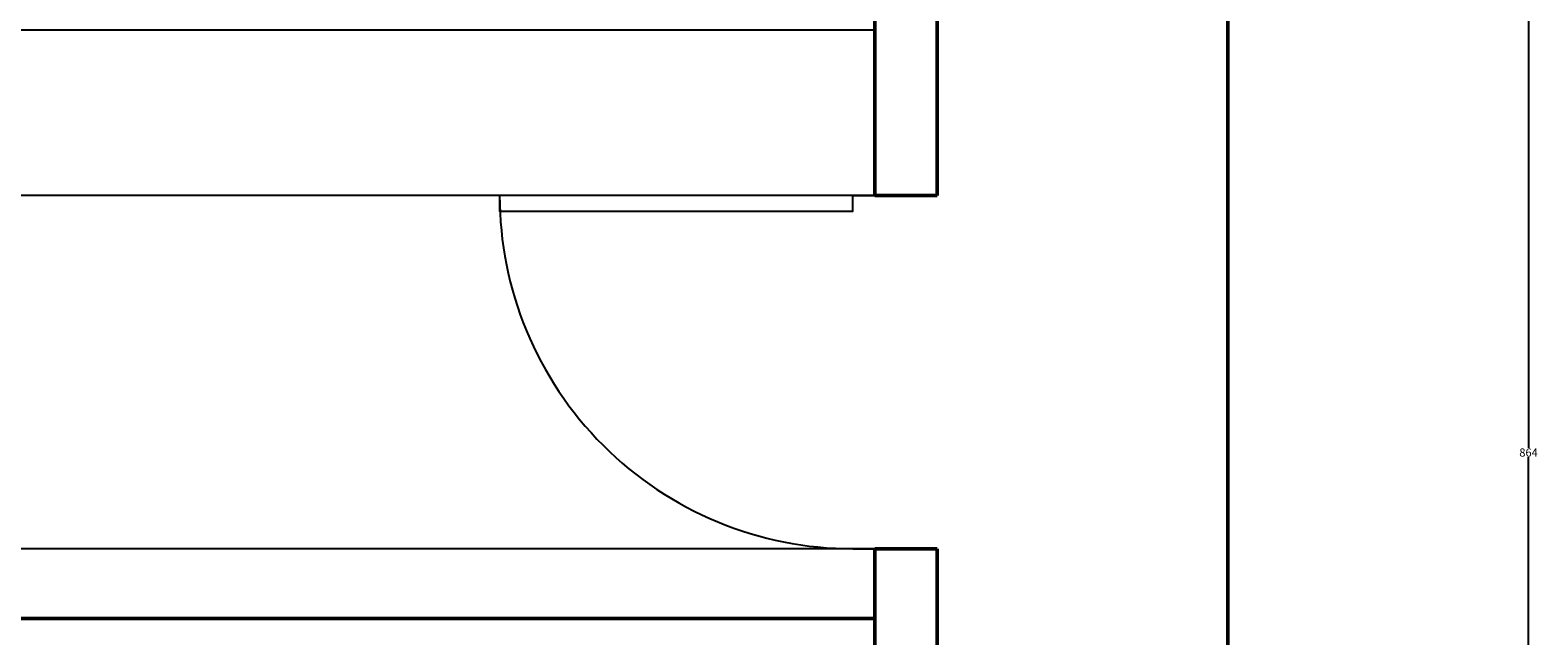
# Model space of a CAD drawing. Units: inches. Extents: x 3506 to 3958, y 1553 to 2506.
# Tile 11 of 16: x 3739 to 3957, y 2003 to 2090. Entities that reach past the tile are written whole.
import ezdxf

# ---------------------------------------------------------------- set-up
doc = ezdxf.new("R2010")
doc.units = ezdxf.units.IN
doc.header["$MEASUREMENT"] = 0
for name, color, linetype, lineweight in [('A-ANNO-DIMS', 2, 'Continuous', 18), ('A-WALL', 7, 'Continuous', 50), ('doors', 40, 'Continuous', 25)]:
    doc.layers.add(name, color=color, linetype=linetype, lineweight=lineweight)
doc.layers.add('A-WALL-PATT', color=251, linetype='Continuous', lineweight=13, true_color=0x636466)
doc.styles.get("Standard").update_dxf_attribs({"font": 'arial.ttf'})
doc.dimstyles.get("Standard").update_dxf_attribs({"dimtxt": 1.18, "dimasz": 0.68, "dimexe": 0.18, "dimexo": 0.0625, "dimgap": 0.09, "dimtad": 0, "dimtih": 1, "dimtoh": 1, "dimdec": 1, "dimzin": 0, "dimdsep": 46, "dimlunit": 3, "dimtxsty": 'Standard', "dimcen": 0.09, "dimadec": 0, "dimazin": 0, "dimtfac": 1, "dimtdec": 1, "dimtofl": 0, "dimtmove": 0, "dimatfit": 3, "dimfxl": 1, "dimtolj": 1, "dimtzin": 0, "dimarcsym": 0})

# ---------------------------------------------------------------- blocks, each defined once
blk = doc.blocks.new('*U12')
for p, q in [((0, 0), (0, 6)), ((40, 0), (40, 6))]:
    blk.add_line(p, q)
blk.add_lwpolyline([(0, 0), (0, -40), (1.75, -40), (1.75, 0)], close=True)
blk.add_arc((0, 0), 40, 270, 0)
blk = doc.blocks.new('*D39')
at = {"layer": 'A-ANNO-DIMS', "color": 0, "lineweight": -2, "transparency": 16777216}
for p, q in [((3911.79, 2461.39), (3955.36, 2461.39)), ((3955.18, 2460.71), (3955.18, 2030.09)), ((3955.18, 1598.07), (3955.18, 2028.7)), ((3911.79, 1597.39), (3955.36, 1597.39))]:
    blk.add_line(p, q, dxfattribs=at)
at = {"layer": 'A-ANNO-DIMS', "color": 0, "transparency": 16777216}
for points in [[(3955.07, 2460.71), (3955.29, 2460.71), (3955.18, 2461.39)], [(3955.07, 1598.07), (3955.29, 1598.07), (3955.18, 1597.39)]]:
    blk.add_solid(points, dxfattribs=at)
at = {"layer": 'Defpoints', "color": 0, "transparency": 16777216}
for p in [(3911.73, 2461.39), (3955.18, 2461.39), (3911.73, 1597.39)]:
    blk.add_point(p, dxfattribs=at)
at = {"layer": 'A-ANNO-DIMS', "color": 0, "transparency": 16777216, "insert": (3955.18, 2029.39), "char_height": 1.18, "attachment_point": 5}
blk.add_mtext('\\A1;864', dxfattribs=at)
blk = doc.blocks.new('*D60')
at = {"layer": 'A-ANNO-DIMS', "color": 0, "lineweight": -2, "transparency": 16777216}
for p, q in [((3860.67, 2066.52), (3508.1, 2066.52)), ((3508.28, 2065.84), (3508.28, 2041.7)), ((3508.28, 2016.17), (3508.28, 2040.31)), ((3860.67, 2015.49), (3508.1, 2015.49))]:
    blk.add_line(p, q, dxfattribs=at)
at = {"layer": 'A-ANNO-DIMS', "color": 0, "transparency": 16777216}
for points in [[(3508.17, 2065.84), (3508.39, 2065.84), (3508.28, 2066.52)], [(3508.17, 2016.17), (3508.39, 2016.17), (3508.28, 2015.49)]]:
    blk.add_solid(points, dxfattribs=at)
at = {"layer": 'Defpoints', "color": 0, "transparency": 16777216}
for p in [(3860.73, 2066.52), (3508.28, 2015.49), (3860.73, 2015.49)]:
    blk.add_point(p, dxfattribs=at)
at = {"layer": 'A-ANNO-DIMS', "color": 0, "transparency": 16777216, "insert": (3508.28, 2041), "char_height": 1.18, "attachment_point": 5}
blk.add_mtext('\\A1;51.03', dxfattribs=at)
blk = doc.blocks.new('*D61')
at = {"layer": 'A-ANNO-DIMS', "color": 0, "lineweight": -2, "transparency": 16777216}
for p, q in [((3860.67, 2090.43), (3508.1, 2090.43)), ((3508.28, 2089.75), (3508.28, 2079.17)), ((3508.28, 2067.2), (3508.28, 2077.78)), ((3860.67, 2066.52), (3508.1, 2066.52))]:
    blk.add_line(p, q, dxfattribs=at)
at = {"layer": 'A-ANNO-DIMS', "color": 0, "transparency": 16777216}
for points in [[(3508.17, 2089.75), (3508.39, 2089.75), (3508.28, 2090.43)], [(3508.17, 2067.2), (3508.39, 2067.2), (3508.28, 2066.52)]]:
    blk.add_solid(points, dxfattribs=at)
at = {"layer": 'Defpoints', "color": 0, "transparency": 16777216}
for p in [(3860.73, 2090.43), (3508.28, 2066.52), (3860.73, 2066.52)]:
    blk.add_point(p, dxfattribs=at)
at = {"layer": 'A-ANNO-DIMS', "color": 0, "transparency": 16777216, "insert": (3508.28, 2078.48), "char_height": 1.18, "attachment_point": 5}
blk.add_mtext('\\A1;23.92', dxfattribs=at)

msp = doc.modelspace()

# ---------------------------------------------------------------- hatches: boundary and pattern name
at = {"layer": 'A-WALL-PATT'}
h = msp.add_hatch(dxfattribs=at)
h.set_pattern_fill('ANSI31', color=256)
h.paths.add_polyline_path([(3911.7302, 2461.3942), (3551.7302, 2461.3942), (3551.7302, 2152.516), (3560.7302, 2152.516), (3560.7302, 2116.516), (3551.7302, 2116.516), (3551.7302, 1920.5711), (3556.2302, 1920.5711), (3560.7302, 1920.5711), (3560.7302, 2000.3942), (3692.7302, 2000.3942), (3692.7302, 1997.3942), (3697.7302, 1997.3942), (3697.7302, 2000.3942), (3771.7302, 2000.3942), (3771.7302, 1997.3942), (3776.7302, 1997.3942), (3776.7302, 1997.7206), (3778.5802, 1997.7206), (3807.5802, 1997.7206), (3807.5802, 1996.4519), (3778.5802, 1996.4519), (3778.5802, 1997.7206), (3776.7302, 1997.7206), (3776.7302, 1997.3942), (3771.7302, 1997.3942), (3771.7302, 2000.3942), (3697.7302, 2000.3942), (3697.7302, 1997.3942), (3692.7302, 1997.3942), (3689.8302, 1997.3942), (3689.8302, 1995.8192), (3653.8302, 1995.8192), (3653.8302, 1997.3942), (3689.8302, 1997.3942), (3692.7302, 1997.3942), (3692.7302, 2000.3942), (3560.7302, 2000.3942), (3560.7302, 1920.5711), (3551.7302, 1920.5711), (3551.7302, 1884.5711), (3551.7302, 1597.3942), (3911.7302, 1597.3942)], flags=17)
h.paths.add_polyline_path([(3596.7302, 2005.3942), (3596.7302, 2057.3035, -0.38730371), (3569.1778, 2085), (3569.15, 2085), (3569.15, 2086.2688), (3598.15, 2086.2688), (3598.15, 2085), (3569.1778, 2085, 0.38730371), (3596.7302, 2057.3035), (3596.7302, 2057.3942), (3601.7302, 2057.3942), (3601.7302, 2055.3942), (3630.7302, 2055.3942), (3630.7302, 2034.3942), (3694.7302, 2034.3942), (3694.7302, 2053.3942), (3699.7302, 2053.3942), (3699.7302, 2005.3942), (3860.7302, 2005.3942), (3860.7302, 2173.3942), (3771.7302, 2173.3942), (3771.7302, 2194.3942), (3776.7302, 2194.3942), (3776.7302, 2178.3942), (3860.7302, 2178.3942), (3860.7302, 2231.3942), (3601.7302, 2231.3942), (3601.7302, 2241.426), (3596.7302, 2241.426), (3596.7302, 2231.3942), (3560.7302, 2231.3942), (3560.7302, 2315.3942), (3596.7302, 2315.3942), (3596.7302, 2312.3942), (3601.7302, 2312.3942), (3601.7302, 2315.3942), (3697.7302, 2315.3942), (3697.7302, 2413.3942), (3692.7302, 2413.3942), (3692.7302, 2320.3942), (3560.7302, 2320.3942), (3560.7302, 2452.3942), (3692.7302, 2452.3942), (3692.7302, 2449.3942), (3697.7302, 2449.3942), (3697.7302, 2452.3942), (3771.7302, 2452.3942), (3771.7302, 2449.3942), (3776.7302, 2449.3942), (3776.7302, 2452.3942), (3860.7302, 2452.3942), (3860.7302, 2437.2075), (3865.2302, 2437.2075), (3865.2302, 2413.2075), (3860.7302, 2413.2075), (3860.7302, 2367.6976), (3865.2302, 2367.6976), (3869.7302, 2367.6976), (3869.7302, 2319.6976), (3860.7302, 2319.6976), (3860.7302, 2211.6248), (3869.7302, 2211.6248), (3869.7302, 2187.6248), (3860.7302, 2187.6248), (3860.7302, 2138.4346), (3865.2302, 2138.4346), (3869.7302, 2138.4346), (3869.7302, 2090.4346), (3860.7302, 2090.4346), (3860.7302, 1985.8449), (3869.7302, 1985.8449), (3869.7302, 1961.8449), (3860.7302, 1961.8449), (3860.7302, 1897.0756), (3865.2302, 1897.0756), (3869.7302, 1897.0756), (3869.7302, 1849.0756), (3860.7302, 1849.0756), (3860.7302, 1847.8112), (3860.7302, 1779.3942), (3596.7302, 1779.3942), (3596.7302, 1831.3942), (3601.7302, 1831.3942), (3601.7302, 1828.3942), (3630.7302, 1828.3942), (3630.7302, 1808.3942), (3691.7302, 1808.3942), (3691.7302, 1815.3942), (3696.7302, 1815.3942), (3696.7302, 1779.3942), (3860.7302, 1779.3942), (3860.7302, 1947.3942), (3771.7302, 1947.3942), (3771.7302, 1968.3942), (3776.7302, 1968.3942), (3776.7302, 1952.3942), (3860.7302, 1952.3942), (3860.7302, 2005.3942)], flags=0)
h.paths.add_polyline_path([(3596.7302, 2038.8546), (3601.7302, 2038.8546), (3601.7302, 2014.8546), (3596.7302, 2014.8546)], flags=0)
h.paths.add_polyline_path([(3564.1688, 2107), (3564.1688, 2167), (3644.1688, 2167), (3644.1688, 2107)], flags=0)
h.paths.add_polyline_path([(3607.0972, 2052.0208), (3620.8472, 2052.0208, -0.41421356), (3621.9931, 2050.875), (3621.9931, 2025.6667, -0.41421356), (3620.8472, 2024.5208), (3607.0972, 2024.5208, -0.41421356), (3605.9514, 2025.6667), (3605.9514, 2050.875, -0.41421356)], flags=0)
h.paths.add_polyline_path([(3578.5688, 2115), (3565.3688, 2115), (3565.3688, 2135.8), (3578.5688, 2135.8), (3578.5688, 2138.2), (3565.3688, 2138.2), (3565.3688, 2159), (3580.5688, 2159), (3580.5688, 2153.8), (3593.7688, 2167), (3593.7688, 2151.8), (3578.5688, 2151.8)], flags=0)
h.paths.add_polyline_path([(3610.9167, 2050.875), (3620.0833, 2050.875, -0.41421356), (3620.8472, 2050.1111), (3620.8472, 2039.6076, -0.41421356), (3620.0833, 2038.8438), (3610.9167, 2038.8438, -0.41421356), (3610.1528, 2039.6076), (3610.1528, 2050.1111, -0.41421356)], flags=0)
h.paths.add_polyline_path([(3610.9167, 2037.6979), (3620.0833, 2037.6979, -0.41421356), (3620.8472, 2036.934), (3620.8472, 2026.4306, -0.41421356), (3620.0833, 2025.6667), (3610.9167, 2025.6667, -0.41421356), (3610.1528, 2026.4306), (3610.1528, 2036.934, -0.41421356)], flags=0)
h.paths.add_polyline_path([(3616.2639, 2044.7639, -1), (3614.7361, 2044.7639, -1)], flags=0)
h.paths.add_polyline_path([(3615.8819, 2044.7639, -1), (3615.1181, 2044.7639, -1)], flags=0)
h.paths.add_polyline_path([(3616.2639, 2031.7778, -1), (3614.7361, 2031.7778, -1)], flags=0)
h.paths.add_polyline_path([(3615.8819, 2031.7778, -1), (3615.1181, 2031.7778, -1)], flags=0)
h.paths.add_polyline_path([(3609.7539, 2021.7868), (3626.9586, 2021.7868), (3626.9586, 2008.8833), (3609.7539, 2008.8833)], flags=0)
h.paths.add_polyline_path([(3610.4708, 2021.07), (3621.2237, 2021.07), (3621.2237, 2009.6002), (3610.4708, 2009.6002)], flags=0)
h.paths.add_polyline_path([(3611.5461, 2019.9947), (3620.1484, 2019.9947), (3620.1484, 2010.6755), (3611.5461, 2010.6755)], flags=0)
h.paths.add_polyline_path([(3621.9405, 2021.07), (3626.2417, 2021.07), (3626.2417, 2009.6002), (3621.9405, 2009.6002)], flags=0)
h.paths.add_polyline_path([(3622.6574, 2020.3531), (3625.5248, 2020.3531), (3625.5248, 2017.4857), (3622.6574, 2017.4857)], flags=0)
h.paths.add_polyline_path([(3622.6574, 2016.7688), (3625.5248, 2016.7688), (3625.5248, 2010.317), (3622.6574, 2010.317)], flags=0)
h.paths.add_polyline_path([(3624.808, 2016.0519), (3624.808, 2013.9013), (3624.0911, 2013.9013), (3624.0911, 2013.1845), (3623.3743, 2013.1845), (3623.3743, 2013.9013), (3623.3743, 2016.0519)], flags=0)
h.paths.add_polyline_path([(3623.0158, 2012.8261), (3625.1664, 2012.8261), (3625.1664, 2012.1092), (3623.0158, 2012.1092)], flags=0)
h.paths.add_polyline_path([(3623.0158, 2011.7508), (3625.1664, 2011.7508), (3625.1664, 2011.0339), (3623.0158, 2011.0339)], flags=0)
h.paths.add_polyline_path([(3650.0591, 2031.8202), (3674.0368, 2031.8202), (3674.0368, 2012.638), (3669.2413, 2012.638), (3669.2413, 2011.8388), (3672.4383, 2011.8388), (3672.4383, 2011.0395), (3651.6576, 2011.0395), (3651.6576, 2011.8388), (3654.8546, 2011.8388), (3654.8546, 2012.638), (3650.0591, 2012.638)], flags=0)
h.paths.add_polyline_path([(3658.0517, 2024.6269, -1), (3651.6576, 2024.6269, -1)], flags=0)
h.paths.add_polyline_path([(3657.2524, 2024.6269, -1), (3652.4569, 2024.6269, -1)], flags=0)
h.paths.add_polyline_path([(3656.4532, 2024.6269, -1), (3653.2561, 2024.6269, -1)], flags=0)
h.paths.add_polyline_path([(3655.6539, 2024.6269, -1), (3654.0554, 2024.6269, -1)], flags=0)
h.paths.add_polyline_path([(3657.2524, 2017.4336, -1), (3652.4569, 2017.4336, -1)], flags=0)
h.paths.add_polyline_path([(3656.4532, 2017.4336, -1), (3653.2561, 2017.4336, -1)], flags=0)
h.paths.add_polyline_path([(3655.6539, 2017.4336, -1), (3654.0554, 2017.4336, -1)], flags=0)
h.paths.add_polyline_path([(3659.6502, 2027.8239), (3664.4457, 2027.8239), (3664.4457, 2015.0358), (3659.6502, 2015.0358)], flags=0)
h.paths.add_polyline_path([(3663.6465, 2027.0247), (3663.6465, 2015.8351), (3660.4494, 2015.8351), (3660.4494, 2027.0247)], flags=0)
h.paths.add_polyline_path([(3562.6688, 1945.5), (3642.6688, 1945.5), (3642.6688, 1885.5), (3562.6688, 1885.5)], flags=0)
h.paths.add_polyline_path([(3671.6391, 2024.6269, -1), (3666.8435, 2024.6269, -1)], flags=0)
h.paths.add_polyline_path([(3670.8398, 2024.6269, -1), (3667.6428, 2024.6269, -1)], flags=0)
h.paths.add_polyline_path([(3672.4383, 2017.4336, -1), (3666.0443, 2017.4336, -1)], flags=0)
h.paths.add_polyline_path([(3670.0405, 2024.6269, -1), (3668.442, 2024.6269, -1)], flags=0)
h.paths.add_polyline_path([(3671.6391, 2017.4336, -1), (3666.8435, 2017.4336, -1)], flags=0)
h.paths.add_polyline_path([(3670.8398, 2017.4336, -1), (3667.6428, 2017.4336, -1)], flags=0)
h.paths.add_polyline_path([(3592.2688, 1945.5), (3592.2688, 1930.3), (3577.0688, 1930.3), (3577.0688, 1893.5), (3563.8688, 1893.5), (3563.8688, 1914.3), (3577.0688, 1914.3), (3577.0688, 1916.7), (3563.8688, 1916.7), (3563.8688, 1937.5), (3579.0688, 1937.5), (3579.0688, 1932.3)], flags=0)
h.paths.add_polyline_path([(3670.0405, 2017.4336, -1), (3668.442, 2017.4336, -1)], flags=0)
h.paths.add_polyline_path([(3596.7302, 2283.3942), (3601.7302, 2283.3942), (3601.7302, 2265.426), (3599.2302, 2265.426), (3599.2302, 2241.426), (3596.7302, 2241.426), (3596.7302, 2265.426)], flags=0)
h.paths.add_polyline_path([(3596.7302, 1810.7006), (3601.7302, 1810.7006), (3601.7302, 1786.7006), (3596.7302, 1786.7006)], flags=0)
h.paths.add_polyline_path([(3560.7302, 1770.3942), (3738.7302, 1770.3942), (3738.7302, 1746.3942), (3738.7302, 1722.3942), (3748.7302, 1722.3942), (3748.7302, 1674.3942), (3560.7302, 1674.3942)], flags=0)
h.paths.add_polyline_path([(3728.7302, 1746.3942), (3728.7302, 1756.0642), (3738.7302, 1746.3942), (3728.7302, 1738.1582), (3728.7302, 1698.3942), (3591.2519, 1698.3942), (3591.2519, 1746.3942)], flags=0)
h.paths.add_polyline_path([(3771.7302, 2399.3942), (3771.7302, 2420.3942), (3776.7302, 2420.3942), (3776.7302, 2404.3942), (3776.7302, 2399.3942)], flags=0)
h.paths.add_polyline_path([(3911.7302, 2461.3942), (3551.7302, 2461.3942), (3551.7302, 2152.516), (3560.7302, 2152.516), (3560.7302, 2116.516), (3551.7302, 2116.516), (3551.7302, 1920.5711), (3560.7302, 1920.5711), (3560.7302, 2000.3942), (3692.7302, 2000.3942), (3692.7302, 1997.3942), (3697.7302, 1997.3942), (3697.7302, 2000.3942), (3771.7302, 2000.3942), (3771.7302, 1997.3942), (3776.7302, 1997.3942), (3776.7302, 1997.7206), (3778.5802, 1997.7206), (3807.5802, 1997.7206), (3807.5802, 1996.4519), (3778.5802, 1996.4519), (3778.5802, 1997.7206), (3776.7302, 1997.7206), (3776.7302, 1997.3942), (3771.7302, 1997.3942), (3771.7302, 2000.3942), (3697.7302, 2000.3942), (3697.7302, 1997.3942), (3692.7302, 1997.3942), (3689.8302, 1997.3942), (3689.8302, 1995.8192), (3653.8302, 1995.8192), (3653.8302, 1997.3942), (3689.8302, 1997.3942), (3692.7302, 1997.3942), (3692.7302, 2000.3942), (3560.7302, 2000.3942), (3560.7302, 1920.5711), (3551.7302, 1920.5711), (3551.7302, 1597.3942), (3911.7302, 1597.3942)], flags=17)

# ---------------------------------------------------------------- linework, layer by layer
at = {"layer": 'A-WALL'}
for p, q in [((3860.7302, 2249.8816), (3860.7302, 2066.516)), ((3869.7302, 2249.8816), (3869.7302, 2066.516)), ((3860.7302, 2066.516), (3869.7302, 2066.516)), ((3869.7302, 2015.4906), (3860.7302, 2015.4906)), ((3860.7302, 2015.4906), (3860.7302, 1838.7087)), ((3869.7302, 2015.4906), (3869.7302, 1838.7087)), ((3560.7302, 2005.3942), (3860.7302, 2005.3942))]:
    msp.add_line(p, q, dxfattribs=at)
msp.add_lwpolyline([(3551.7302, 2461.3942), (3911.7302, 2461.3942), (3911.7302, 1597.3942), (3551.7302, 1597.3942)], close=True, dxfattribs=at)

# ---------------------------------------------------------------- block references
at = {"layer": 'doors', "xscale": 1.27563568336709, "yscale": 1.27563568336709, "zscale": 1.27563568336709, "rotation": 270}
msp.add_blockref('*U12', (3857.5764, 2066.516), dxfattribs=at)

# ---------------------------------------------------------------- dimensions: what is measured, and where the dimension line sits
at = {"layer": 'A-ANNO-DIMS'}
for base, p1, p2, override, picture, middle in [((3955.1802, 2461.3942), (3911.7302, 1597.3942), (3911.7302, 2461.3942), {"dimdec": 0, "dimlfac": 1, "dimrnd": 0, "dimzin": 0, "dimdsep": 46, "dimlunit": 2}, '*D39', (3955.1802, 2029.3942)), ((3508.2802, 2066.516), (3860.7302, 2090.4346), (3860.7302, 2066.516), {"dimdec": 2, "dimlfac": 1, "dimrnd": 0, "dimzin": 0, "dimdsep": 46, "dimlunit": 2}, '*D61', (3508.2802, 2078.4753)), ((3508.2802, 2015.4906), (3860.7302, 2066.516), (3860.7302, 2015.4906), {"dimdec": 2, "dimlfac": 1, "dimrnd": 0, "dimzin": 0, "dimdsep": 46, "dimlunit": 2}, '*D60', (3508.2802, 2041.0033))]:
    dim = msp.add_linear_dim(base=base, p1=p1, p2=p2, angle=90, dimstyle='Standard', override=override, dxfattribs=at)
    dim.commit()
    dim.dimension.update_dxf_attribs({"geometry": picture, "text_midpoint": middle})

doc.saveas('drawing.dxf')
